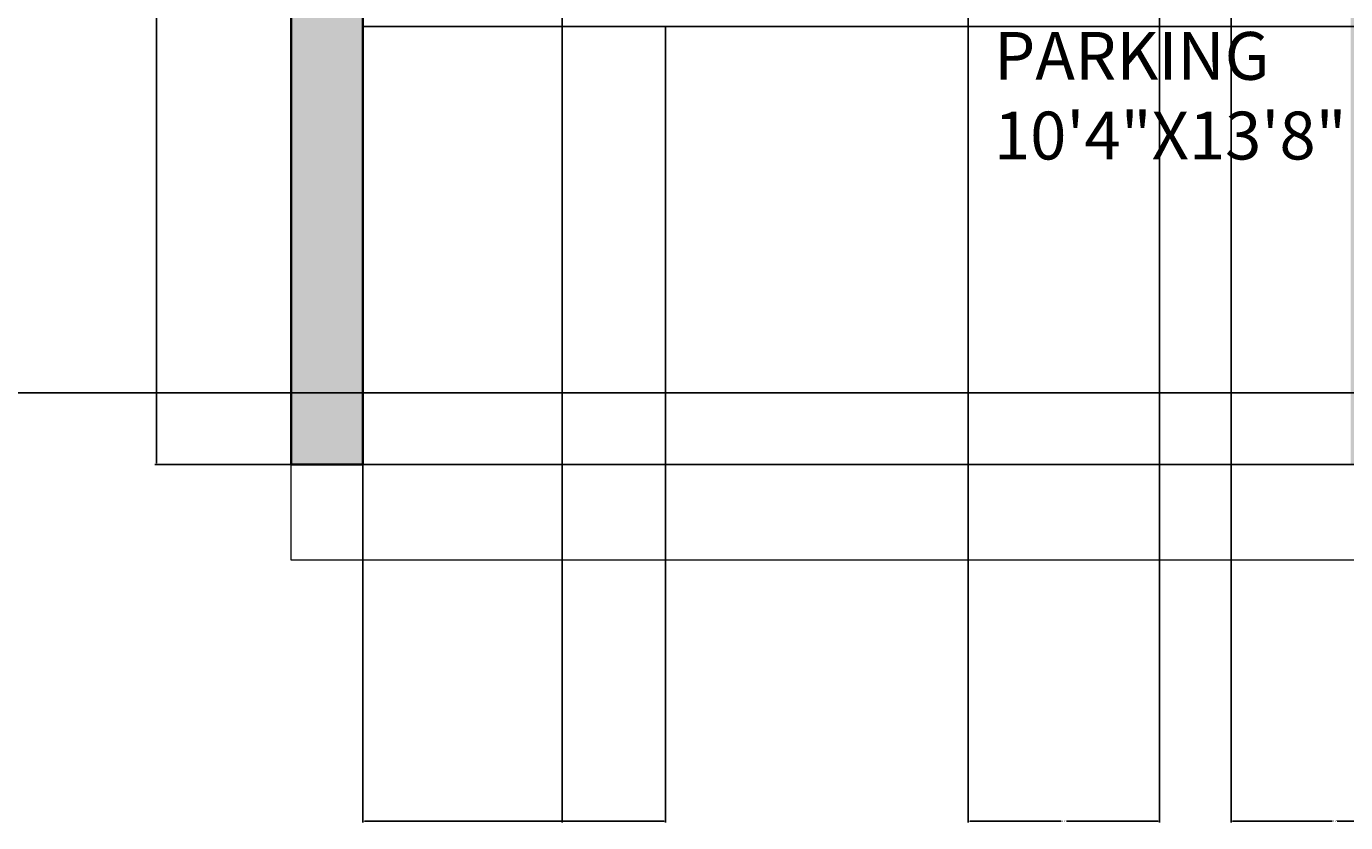
# Model space of a CAD drawing. Units: inches. Extents: x 37 to 706, y -568 to 110.
# Tile 9 of 24: x 361 to 526, y -568 to -468. Entities that reach past the tile are written whole.
import ezdxf

# ---------------------------------------------------------------- set-up
doc = ezdxf.new("R2010")
doc.units = ezdxf.units.IN
doc.header["$MEASUREMENT"] = 0
for name, color, linetype, lineweight in [('A-ANNO-DIMS', 2, 'Continuous', 18), ('A-AREA-IDEN', 7, 'Continuous', 18), ('A-FLOR-STRS', 7, 'Continuous', 18), ('A-WALL', 7, 'Continuous', 35), ('A-WALL-PATT', 252, 'Continuous', 13)]:
    doc.layers.add(name, color=color, linetype=linetype, lineweight=lineweight)
doc.styles.get("Standard").update_dxf_attribs({"font": 'arial.ttf'})
doc.dimstyles.get("Standard").update_dxf_attribs({"dimtxt": 0.18, "dimasz": 0.18, "dimexe": 0.18, "dimexo": 0.0625, "dimgap": 0.09, "dimtad": 0, "dimtih": 1, "dimtoh": 1, "dimdec": 0, "dimzin": 0, "dimdsep": 46, "dimlunit": 3, "dimtxsty": 'Standard', "dimcen": 0.09, "dimadec": 0, "dimazin": 0, "dimtfac": 1, "dimtdec": 0, "dimtofl": 0, "dimtmove": 0, "dimatfit": 3, "dimfxl": 1, "dimtolj": 1, "dimtzin": 0, "dimarcsym": 0})

# ---------------------------------------------------------------- blocks, each defined once
blk = doc.blocks.new('*D5')
at = {"layer": 'A-ANNO-DIMS', "color": 0, "lineweight": -2, "transparency": 16777216}
for p, q in [((393.9, 51.29), (376.84, 51.29)), ((377.02, 51.11), (377.02, -232.56)), ((377.02, -522.53), (377.02, -238.86)), ((393.9, -522.71), (376.84, -522.71))]:
    blk.add_line(p, q, dxfattribs=at)
at = {"layer": 'A-ANNO-DIMS', "color": 0, "transparency": 16777216}
for points in [[(376.99, 51.11), (377.05, 51.11), (377.02, 51.29)], [(376.99, -522.53), (377.05, -522.53), (377.02, -522.71)]]:
    blk.add_solid(points, dxfattribs=at)
at = {"layer": 'Defpoints', "color": 0, "transparency": 16777216}
for p in [(393.96, 51.29), (377.02, -522.71), (393.96, -522.71)]:
    blk.add_point(p, dxfattribs=at)
at = {"layer": 'A-ANNO-DIMS', "color": 0, "transparency": 16777216, "insert": (377.02, -235.71), "char_height": 6, "attachment_point": 5}
blk.add_mtext('\\A1;47\'-10"', dxfattribs=at)
blk = doc.blocks.new('ENTRY-STEP-236')
for p, q in [((0, 0), (0, 12)), ((236, 0), (0, 0))]:
    blk.add_line(p, q)
blk = doc.blocks.new('*D44')
at = {"layer": 'A-ANNO-DIMS', "color": 0, "lineweight": -2, "transparency": 16777216}
for p, q in [((402.96, -467.77), (402.96, -567.64)), ((440.96, -467.77), (440.96, -567.64)), ((403.14, -567.46), (421.63, -567.46)), ((440.78, -567.46), (422.29, -567.46))]:
    blk.add_line(p, q, dxfattribs=at)
at = {"layer": 'A-ANNO-DIMS', "color": 0, "transparency": 16777216}
for points in [[(403.14, -567.43), (403.14, -567.49), (402.96, -567.46)], [(440.78, -567.43), (440.78, -567.49), (440.96, -567.46)]]:
    blk.add_solid(points, dxfattribs=at)
at = {"layer": 'Defpoints', "color": 0, "transparency": 16777216}
for p in [(402.96, -467.71), (440.96, -467.71), (440.96, -567.46)]:
    blk.add_point(p, dxfattribs=at)
at = {"layer": 'A-ANNO-DIMS', "color": 0, "transparency": 16777216, "insert": (421.96, -567.46), "char_height": 0.18, "attachment_point": 5}
blk.add_mtext('\\A1;3\'-2"', dxfattribs=at)
blk = doc.blocks.new('*D45')
at = {"layer": 'A-ANNO-DIMS', "color": 0, "lineweight": -2, "transparency": 16777216}
for p, q in [((88.02, -449.71), (705.89, -449.71)), ((705.71, -449.89), (705.71, -481.53)), ((705.71, -513.53), (705.71, -481.89)), ((79.02, -513.71), (705.89, -513.71))]:
    blk.add_line(p, q, dxfattribs=at)
at = {"layer": 'A-ANNO-DIMS', "color": 0, "transparency": 16777216}
for points in [[(705.68, -449.89), (705.74, -449.89), (705.71, -449.71)], [(705.68, -513.53), (705.74, -513.53), (705.71, -513.71)]]:
    blk.add_solid(points, dxfattribs=at)
at = {"layer": 'Defpoints', "color": 0, "transparency": 16777216}
for p in [(87.96, -449.71), (705.71, -449.71), (78.96, -513.71)]:
    blk.add_point(p, dxfattribs=at)
at = {"layer": 'A-ANNO-DIMS', "color": 0, "transparency": 16777216, "insert": (705.71, -481.71), "char_height": 0.18, "attachment_point": 5}
blk.add_mtext('\\A1;5\'-4"', dxfattribs=at)
blk = doc.blocks.new('*D46')
at = {"layer": 'A-ANNO-DIMS', "color": 0, "lineweight": -2, "transparency": 16777216}
for p, q in [((403.020833, -467.708464), (705.888333, -467.708464)), ((705.708333, -467.888464), (705.708333, -495.028464)), ((705.708333, -522.528464), (705.708333, -495.388464)), ((394.020833, -522.708464), (705.888333, -522.708464))]:
    blk.add_line(p, q, dxfattribs=at)
at = {"layer": 'A-ANNO-DIMS', "color": 0, "transparency": 16777216}
for points in [[(705.678333, -467.888464), (705.738333, -467.888464), (705.708333, -467.708464)], [(705.678333, -522.528464), (705.738333, -522.528464), (705.708333, -522.708464)]]:
    blk.add_solid(points, dxfattribs=at)
at = {"layer": 'Defpoints', "color": 0, "transparency": 16777216}
for p in [(402.958333, -467.708464), (705.708333, -467.708464), (393.958333, -522.708464)]:
    blk.add_point(p, dxfattribs=at)
at = {"layer": 'A-ANNO-DIMS', "color": 0, "transparency": 16777216, "insert": (705.708333, -495.208464), "char_height": 0.18, "attachment_point": 5}
blk.add_mtext('\\A1;4\'-7"', dxfattribs=at)
blk = doc.blocks.new('*D53')
at = {"layer": 'A-ANNO-DIMS', "color": 0, "lineweight": -2, "transparency": 16777216}
for p, q in [((511.96, -151.77), (511.96, -567.64)), ((537.96, -151.77), (537.96, -567.64)), ((512.14, -567.46), (524.63, -567.46)), ((537.78, -567.46), (525.29, -567.46))]:
    blk.add_line(p, q, dxfattribs=at)
at = {"layer": 'A-ANNO-DIMS', "color": 0, "transparency": 16777216}
for points in [[(512.14, -567.43), (512.14, -567.49), (511.96, -567.46)], [(537.78, -567.43), (537.78, -567.49), (537.96, -567.46)]]:
    blk.add_solid(points, dxfattribs=at)
at = {"layer": 'Defpoints', "color": 0, "transparency": 16777216}
for p in [(511.96, -151.71), (537.96, -151.71), (537.96, -567.46)]:
    blk.add_point(p, dxfattribs=at)
at = {"layer": 'A-ANNO-DIMS', "color": 0, "transparency": 16777216, "insert": (524.96, -567.46), "char_height": 0.18, "attachment_point": 5}
blk.add_mtext('\\A1;2\'-2"', dxfattribs=at)
blk = doc.blocks.new('*D56')
at = {"layer": 'A-ANNO-DIMS', "color": 0, "lineweight": -2, "transparency": 16777216}
for p, q in [((402.96, -142.77), (402.96, -567.64)), ((427.97, -142.77), (427.97, -567.64)), ((403.14, -567.46), (415.13, -567.46)), ((427.79, -567.46), (415.79, -567.46))]:
    blk.add_line(p, q, dxfattribs=at)
at = {"layer": 'A-ANNO-DIMS', "color": 0, "transparency": 16777216}
for points in [[(403.14, -567.43), (403.14, -567.49), (402.96, -567.46)], [(427.79, -567.43), (427.79, -567.49), (427.97, -567.46)]]:
    blk.add_solid(points, dxfattribs=at)
at = {"layer": 'Defpoints', "color": 0, "transparency": 16777216}
for p in [(402.96, -142.71), (427.97, -142.71), (427.97, -567.46)]:
    blk.add_point(p, dxfattribs=at)
at = {"layer": 'A-ANNO-DIMS', "color": 0, "transparency": 16777216, "insert": (415.46, -567.46), "char_height": 0.18, "attachment_point": 5}
blk.add_mtext('\\A1;2\'-1"', dxfattribs=at)
blk = doc.blocks.new('*D63')
at = {"layer": 'A-ANNO-DIMS', "color": 0, "lineweight": -2, "transparency": 16777216}
for p, q in [((478.96, -142.77), (478.96, -567.64)), ((502.96, -151.77), (502.96, -567.64)), ((479.14, -567.46), (490.63, -567.46)), ((502.78, -567.46), (491.29, -567.46))]:
    blk.add_line(p, q, dxfattribs=at)
at = {"layer": 'A-ANNO-DIMS', "color": 0, "transparency": 16777216}
for points in [[(479.14, -567.43), (479.14, -567.49), (478.96, -567.46)], [(502.78, -567.43), (502.78, -567.49), (502.96, -567.46)]]:
    blk.add_solid(points, dxfattribs=at)
at = {"layer": 'Defpoints', "color": 0, "transparency": 16777216}
for p in [(478.96, -142.71), (502.96, -151.71), (502.96, -567.46)]:
    blk.add_point(p, dxfattribs=at)
at = {"layer": 'A-ANNO-DIMS', "color": 0, "transparency": 16777216, "insert": (490.96, -567.46), "char_height": 0.18, "attachment_point": 5}
blk.add_mtext('\\A1;2\'-0"', dxfattribs=at)

msp = doc.modelspace()

# ---------------------------------------------------------------- hatches: boundary and pattern name
at = {"layer": 'A-WALL-PATT'}
h = msp.add_hatch(color=256, dxfattribs=at)
h.dxf.hatch_style = 1
h.paths.add_polyline_path([(220.96, -351.71), (211.96, -351.71), (211.96, -513.71), (254.96, -513.71), (254.96, -504.71), (220.96, -504.71)], flags=17)
h.paths.add_polyline_path([(220.96, -294.71), (211.96, -294.71), (211.96, -303.71), (220.96, -303.71)], flags=17)
h.paths.add_polyline_path([(175.96, -294.71), (155.87, -294.71), (155.87, -303.71), (155.96, -303.71), (175.96, -303.71)], flags=17)
h.paths.add_polyline_path([(220.96, -16.71), (211.96, -16.71), (211.96, -142.71), (220.96, -142.71)], flags=17)
h.paths.add_polyline_path([(357.96, 51.29), (78.96, 51.29), (78.96, -513.71), (87.96, -513.71), (87.96, -303.71), (95.87, -303.71), (95.87, -294.71), (87.96, -294.71), (87.96, -142.71), (187.96, -142.71), (187.96, -133.71), (87.96, -133.71), (87.96, -25.71), (106.96, -25.71), (106.96, -16.71), (87.96, -16.71), (87.96, 42.29), (348.96, 42.29), (348.96, 17.13), (348.96, -133.71), (246.96, -133.71), (246.96, -142.71), (348.96, -142.71), (348.96, -294.71), (251.96, -294.71), (251.96, -303.71), (348.96, -303.71), (348.96, -351.71), (260.96, -351.71), (260.96, -329.71), (251.96, -329.71), (251.96, -360.71), (327.45, -360.71), (348.96, -360.71), (348.96, -504.71), (314.96, -504.71), (314.96, -513.71), (357.96, -513.71)])
h.paths.add_polyline_path([(416.96, -303.71), (402.96, -303.71), (402.96, -151.71), (478.96, -151.71), (478.96, -142.71), (402.96, -142.71), (402.96, -22.71), (409.96, -22.71), (409.96, -13.71), (402.96, -13.71), (402.96, 42.29), (663.96, 42.29), (663.96, -303.71), (566.96, -303.71), (566.96, -312.71), (663.96, -312.71), (663.96, -360.71), (575.96, -360.71), (575.96, -338.71), (566.96, -338.71), (566.96, -360.71), (566.96, -369.71), (642.45, -369.71), (663.96, -369.71), (663.96, -513.71), (629.96, -513.71), (629.96, -522.71), (672.96, -522.71), (672.96, 51.29), (393.96, 51.29), (393.96, -522.71), (402.96, -522.71), (402.96, -312.71), (416.96, -312.71)])
h.paths.add_polyline_path([(490.96, -303.71), (476.96, -303.71), (476.96, -312.71), (490.96, -312.71)], flags=17)
h.paths.add_polyline_path([(535.96, -303.71), (526.96, -303.71), (526.96, -312.71), (535.96, -312.71)], flags=17)
h.paths.add_polyline_path([(535.96, -369.71), (526.96, -369.71), (526.96, -522.71), (569.96, -522.71), (569.96, -513.71), (535.96, -513.71)], flags=17)
h.paths.add_polyline_path([(511.96, -13.71), (502.96, -13.71), (502.96, -151.71), (511.96, -151.71)], flags=17)
h.paths.add_polyline_path([(651.54, -142.71), (651.54, -120.18), (642.54, -120.18), (642.54, -142.71), (550.54, -142.71), (550.54, -120.71), (541.54, -120.71), (541.54, -142.71), (537.96, -142.71), (537.96, -151.71), (651.54, -151.71)], flags=17)
h.paths.add_polyline_path([(651.54, -85.71), (541.54, -85.71), (541.54, -94.71), (651.54, -94.71)], flags=17)
h.paths.add_polyline_path([(476.96, -13.71), (469.96, -13.71), (469.96, -22.71), (476.96, -22.71)], flags=17)
h.paths.add_polyline_path([(185.96, -16.71), (166.96, -16.71), (166.96, -25.71), (185.96, -25.71)], flags=17)
h.paths.add_polyline_path([(168.91, -414.72), (214.62, -414.72), (214.62, -392.33), (168.91, -392.33)], flags=25)

# ---------------------------------------------------------------- linework, layer by layer
at = {"layer": 'A-WALL'}
for p, q in [((393.96, 51.29), (393.96, -522.71)), ((402.96, -312.71), (402.96, -522.71)), ((393.96, -522.71), (402.96, -522.71))]:
    msp.add_line(p, q, dxfattribs=at)

# ---------------------------------------------------------------- block references
at = {"layer": 'A-FLOR-STRS'}
msp.add_blockref('ENTRY-STEP-236', (393.96, -534.71), dxfattribs=at)

# ---------------------------------------------------------------- texts
at = {"layer": 'A-AREA-IDEN', "insert": (482.19, -468.41), "char_height": 6, "attachment_point": 1}
msp.add_mtext('PARKING\\P10\'4"X13\'8"', dxfattribs=at)

# ---------------------------------------------------------------- dimensions: what is measured, and where the dimension line sits
at = {"layer": 'A-ANNO-DIMS'}
for base, p1, p2, override, picture, middle in [((377.02, -522.71), (393.96, 51.29), (393.96, -522.71), {"dimtxt": 6, "dimclrd": 0, "dimclre": 0, "dimclrt": 0}, '*D5', (377.02, -235.71)), ((705.71, -449.71), (78.96, -513.71), (87.96, -449.71), {"dimdec": 1, "dimlfac": 1, "dimrnd": 0, "dimzin": 1, "dimdsep": 46, "dimlunit": 4, "dimfrac": 2}, '*D45', (705.71, -481.71)), ((705.71, -467.71), (393.96, -522.71), (402.96, -467.71), {"dimdec": 1, "dimlfac": 1, "dimrnd": 0, "dimzin": 1, "dimdsep": 46, "dimlunit": 4, "dimfrac": 2}, '*D46', (705.71, -495.21))]:
    dim = msp.add_linear_dim(base=base, p1=p1, p2=p2, angle=90, dimstyle='Standard', override=override, dxfattribs=at)
    dim.commit()
    dim.dimension.update_dxf_attribs({"geometry": picture, "text_midpoint": middle})
for base, p1, p2, picture, middle in [((427.97, -567.46), (402.96, -142.71), (427.97, -142.71), '*D56', (415.46, -567.46)), ((502.96, -567.46), (478.96, -142.71), (502.96, -151.71), '*D63', (490.96, -567.46)), ((537.96, -567.46), (511.96, -151.71), (537.96, -151.71), '*D53', (524.96, -567.46)), ((440.96, -567.46), (402.96, -467.71), (440.96, -467.71), '*D44', (421.96, -567.46))]:
    dim = msp.add_linear_dim(base=base, p1=p1, p2=p2, dimstyle='Standard', override={"dimdec": 1, "dimlfac": 1, "dimrnd": 0, "dimzin": 1, "dimdsep": 46, "dimlunit": 4, "dimfrac": 2}, dxfattribs=at)
    dim.commit()
    dim.dimension.update_dxf_attribs({"geometry": picture, "text_midpoint": middle})

doc.saveas('drawing.dxf')
